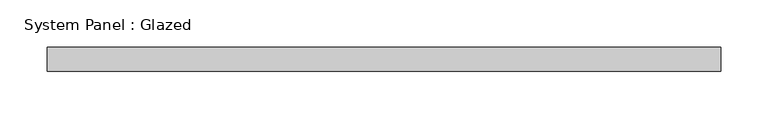
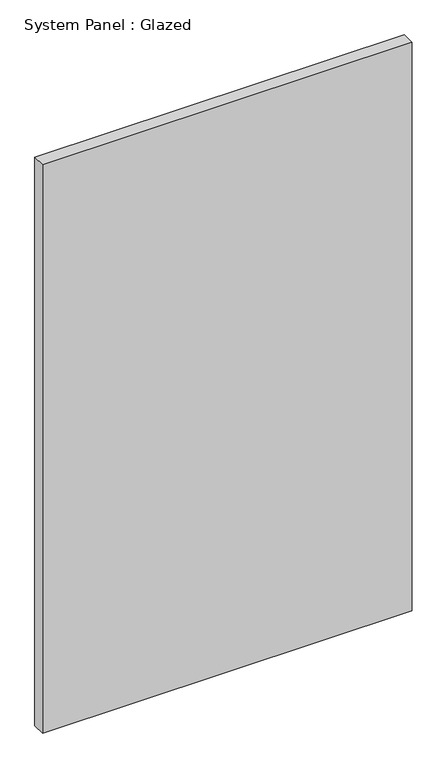
"""IFC4 building model written with IfcOpenShell, lengths in millimetres: plate geometry, System Panel : Glazed."""

from ifc_helpers import new_model, si_unit, origin, origin_with_axes, place, context, project, spatial, polyline, outline, extrude, source, transform, mapped, element, save


def system_panel_glazed_a854efd3(model_context):
    return source(origin(), model_context, "Body", "SweptSolid", [
        extrude(outline(polyline([(355.6, 19.05), (-355.6, 19.05), (-355.6, 44.45), (355.6, 44.45), (355.6, 19.05)])), origin_with_axes(), (0.0, 0.0, 1.0), 1155.7),
    ])


if __name__ == "__main__":
    model = new_model("IFC4")
    model_context = context("Model", 3, world=origin())
    ifc_project = project(units=[si_unit("LENGTHUNIT", "METRE", prefix="MILLI")], contexts=[model_context])
    site = spatial("IfcSite", under=ifc_project)
    building = spatial("IfcBuilding", under=site)
    placement = place(None, origin())
    system_panel_glazed_shape = system_panel_glazed_a854efd3(model_context)
    element("IfcPlate", 1, ObjectType="System Panel : Glazed", at=placement, inside=building, context=model_context, shape_type="MappedRepresentation", body=[
        mapped(system_panel_glazed_shape, transform((0.0, 0.0, 0.0), x_axis=(1.0, 0.0, 0.0), y_axis=(0.0, 1.0, 0.0), z_axis=(0.0, 0.0, 1.0))),
    ])
    save(model, "model.ifc")

# Revit data of these elements
# Type "System Panel : Glazed"
#   Construction Type Id = "GSP4R"
#   Analytic Construction = "1/8 in Pilkington single glazing"
#   Visual Light Transmittance = 0.9
#   Solar Heat Gain Coefficient = 0.86
#   Heat Transfer Coefficient (U) = 1.18115 BTU/(h·ft²·°F)
# Element 1 (IfcPlate, "System Panel : Glazed")
#   Materials on its faces: "Glass"
# Materials
#   "Glass": class "Glass", colour RGB 0 128 192, transparency 0.75, Description = "Soda Lime Glass", Cost = 0
